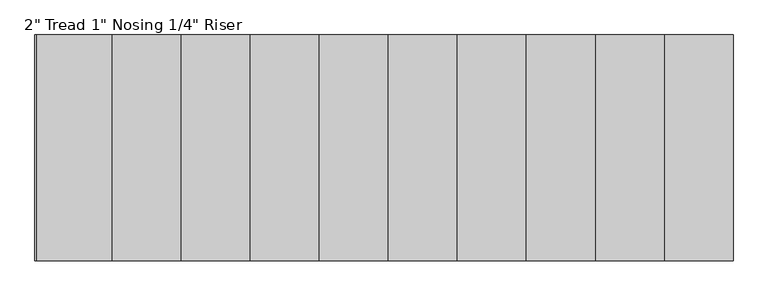
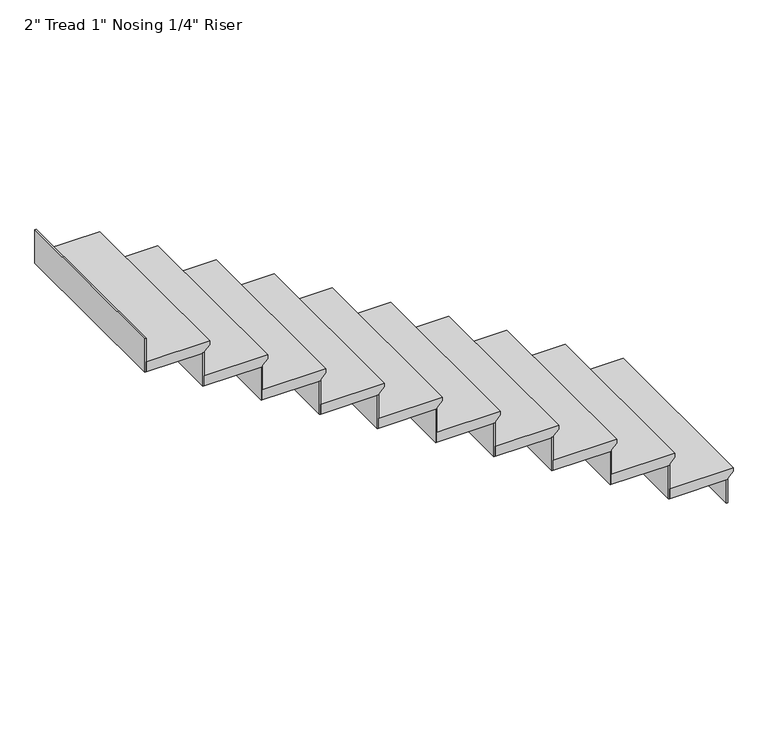
"""IFC4 building model written with IfcOpenShell, lengths in millimetres: stair flight geometry."""

from ifc_helpers import new_model, si_unit, origin, place, context, project, spatial, faceted_brep, source, transform, mapped, element, save


def stair_flight_4502834e(model_context):
    return source(origin(), model_context, "Body", "Brep", [
        faceted_brep([(-5990.8517085, 2919.0826226, 6855.8833333), (-5990.8517085, 2919.0826226, 6874.9333333), (-5990.8517085, 2004.6826226, 6874.9333333), (-5990.8517085, 2004.6826226, 6855.8833333), (-6016.2517085, 2919.0826226, 6830.4833333), (-6016.2517085, 2004.6826226, 6830.4833333), (-6295.6517085, 2919.0826226, 6874.9333333), (-6295.6517085, 2004.6826226, 6874.9333333), (-6016.2517085, 2004.6826226, 6824.1333333), (-6295.6517085, 2004.6826226, 6824.1333333), (-6295.6517085, 2919.0826226, 6824.1333333), (-6016.2517085, 2919.0826226, 6824.1333333)], [[[0, 1, 2, 3]], [[4, 0, 3, 5]], [[2, 1, 6, 7]], [[8, 9, 10, 11]], [[2, 7, 9, 8, 5, 3]], [[8, 11, 4, 5]], [[6, 1, 0, 4, 11, 10]], [[7, 6, 10, 9]]]),
        faceted_brep([(-6016.2517085, 2919.0826226, 6824.1333333), (-6016.2517085, 2919.0826226, 6705.6), (-6022.6017085, 2919.0826226, 6705.6), (-6022.6017085, 2919.0826226, 6824.1333333), (-6016.2517085, 2004.6826226, 6824.1333333), (-6022.6017085, 2004.6826226, 6824.1333333), (-6022.6017085, 2004.6826226, 6705.6), (-6016.2517085, 2004.6826226, 6705.6)], [[[0, 1, 2, 3]], [[4, 5, 6, 7]], [[1, 0, 4, 7]], [[2, 1, 7, 6]], [[3, 2, 6, 5]], [[0, 3, 5, 4]]]),
        faceted_brep([(-6295.6517085, 2919.0826226, 6993.4666667), (-6295.6517085, 2919.0826226, 6824.1333333), (-6302.0017085, 2919.0826226, 6824.1333333), (-6302.0017085, 2919.0826226, 6993.4666667), (-6295.6517085, 2004.6826226, 6993.4666667), (-6302.0017085, 2004.6826226, 6993.4666667), (-6302.0017085, 2004.6826226, 6824.1333333), (-6295.6517085, 2004.6826226, 6824.1333333)], [[[0, 1, 2, 3]], [[4, 5, 6, 7]], [[1, 0, 4, 7]], [[2, 1, 7, 6]], [[3, 2, 6, 5]], [[0, 3, 5, 4]]]),
        faceted_brep([(-6270.2517085, 2004.6826226, 7044.2666667), (-6270.2517085, 2919.0826226, 7044.2666667), (-6575.0517085, 2919.0826226, 7044.2666667), (-6575.0517085, 2004.6826226, 7044.2666667), (-6295.6517085, 2004.6826226, 6993.4666667), (-6575.0517085, 2004.6826226, 6993.4666667), (-6575.0517085, 2919.0826226, 6993.4666667), (-6295.6517085, 2919.0826226, 6993.4666667), (-6295.6517085, 2004.6826226, 6999.8166667), (-6270.2517085, 2004.6826226, 7025.2166667), (-6295.6517085, 2919.0826226, 6999.8166667), (-6270.2517085, 2919.0826226, 7025.2166667)], [[[0, 1, 2, 3]], [[4, 5, 6, 7]], [[0, 3, 5, 4, 8, 9]], [[4, 7, 10, 8]], [[2, 1, 11, 10, 7, 6]], [[3, 2, 6, 5]], [[11, 1, 0, 9]], [[10, 11, 9, 8]]]),
        faceted_brep([(-6575.0517085, 2919.0826226, 7162.8), (-6575.0517085, 2919.0826226, 6993.4666667), (-6581.4017085, 2919.0826226, 6993.4666667), (-6581.4017085, 2919.0826226, 7162.8), (-6575.0517085, 2004.6826226, 7162.8), (-6581.4017085, 2004.6826226, 7162.8), (-6581.4017085, 2004.6826226, 6993.4666667), (-6575.0517085, 2004.6826226, 6993.4666667)], [[[0, 1, 2, 3]], [[4, 5, 6, 7]], [[1, 0, 4, 7]], [[2, 1, 7, 6]], [[3, 2, 6, 5]], [[0, 3, 5, 4]]]),
        faceted_brep([(-6549.6517085, 2004.6826226, 7213.6), (-6549.6517085, 2919.0826226, 7213.6), (-6854.4517085, 2919.0826226, 7213.6), (-6854.4517085, 2004.6826226, 7213.6), (-6575.0517085, 2004.6826226, 7162.8), (-6854.4517085, 2004.6826226, 7162.8), (-6854.4517085, 2919.0826226, 7162.8), (-6575.0517085, 2919.0826226, 7162.8), (-6575.0517085, 2004.6826226, 7169.15), (-6549.6517085, 2004.6826226, 7194.55), (-6575.0517085, 2919.0826226, 7169.15), (-6549.6517085, 2919.0826226, 7194.55)], [[[0, 1, 2, 3]], [[4, 5, 6, 7]], [[0, 3, 5, 4, 8, 9]], [[4, 7, 10, 8]], [[2, 1, 11, 10, 7, 6]], [[3, 2, 6, 5]], [[11, 1, 0, 9]], [[10, 11, 9, 8]]]),
        faceted_brep([(-6854.4517085, 2919.0826226, 7332.1333333), (-6854.4517085, 2919.0826226, 7162.8), (-6860.8017085, 2919.0826226, 7162.8), (-6860.8017085, 2919.0826226, 7332.1333333), (-6854.4517085, 2004.6826226, 7332.1333333), (-6860.8017085, 2004.6826226, 7332.1333333), (-6860.8017085, 2004.6826226, 7162.8), (-6854.4517085, 2004.6826226, 7162.8)], [[[0, 1, 2, 3]], [[4, 5, 6, 7]], [[1, 0, 4, 7]], [[2, 1, 7, 6]], [[3, 2, 6, 5]], [[0, 3, 5, 4]]]),
        faceted_brep([(-6829.0517085, 2004.6826226, 7382.9333333), (-6829.0517085, 2919.0826226, 7382.9333333), (-7133.8517085, 2919.0826226, 7382.9333333), (-7133.8517085, 2004.6826226, 7382.9333333), (-6854.4517085, 2004.6826226, 7332.1333333), (-7133.8517085, 2004.6826226, 7332.1333333), (-7133.8517085, 2919.0826226, 7332.1333333), (-6854.4517085, 2919.0826226, 7332.1333333), (-6854.4517085, 2004.6826226, 7338.4833333), (-6829.0517085, 2004.6826226, 7363.8833333), (-6854.4517085, 2919.0826226, 7338.4833333), (-6829.0517085, 2919.0826226, 7363.8833333)], [[[0, 1, 2, 3]], [[4, 5, 6, 7]], [[0, 3, 5, 4, 8, 9]], [[4, 7, 10, 8]], [[2, 1, 11, 10, 7, 6]], [[3, 2, 6, 5]], [[11, 1, 0, 9]], [[10, 11, 9, 8]]]),
        faceted_brep([(-7133.8517085, 2919.0826226, 7501.4666667), (-7133.8517085, 2919.0826226, 7332.1333333), (-7140.2017085, 2919.0826226, 7332.1333333), (-7140.2017085, 2919.0826226, 7501.4666667), (-7133.8517085, 2004.6826226, 7501.4666667), (-7140.2017085, 2004.6826226, 7501.4666667), (-7140.2017085, 2004.6826226, 7332.1333333), (-7133.8517085, 2004.6826226, 7332.1333333)], [[[0, 1, 2, 3]], [[4, 5, 6, 7]], [[1, 0, 4, 7]], [[2, 1, 7, 6]], [[3, 2, 6, 5]], [[0, 3, 5, 4]]]),
        faceted_brep([(-7108.4517085, 2004.6826226, 7552.2666667), (-7108.4517085, 2919.0826226, 7552.2666667), (-7413.2517085, 2919.0826226, 7552.2666667), (-7413.2517085, 2004.6826226, 7552.2666667), (-7133.8517085, 2004.6826226, 7501.4666667), (-7413.2517085, 2004.6826226, 7501.4666667), (-7413.2517085, 2919.0826226, 7501.4666667), (-7133.8517085, 2919.0826226, 7501.4666667), (-7133.8517085, 2004.6826226, 7507.8166667), (-7108.4517085, 2004.6826226, 7533.2166667), (-7133.8517085, 2919.0826226, 7507.8166667), (-7108.4517085, 2919.0826226, 7533.2166667)], [[[0, 1, 2, 3]], [[4, 5, 6, 7]], [[0, 3, 5, 4, 8, 9]], [[4, 7, 10, 8]], [[2, 1, 11, 10, 7, 6]], [[3, 2, 6, 5]], [[11, 1, 0, 9]], [[10, 11, 9, 8]]]),
        faceted_brep([(-7413.2517085, 2919.0826226, 7670.8), (-7413.2517085, 2919.0826226, 7501.4666667), (-7419.6017085, 2919.0826226, 7501.4666667), (-7419.6017085, 2919.0826226, 7670.8), (-7413.2517085, 2004.6826226, 7670.8), (-7419.6017085, 2004.6826226, 7670.8), (-7419.6017085, 2004.6826226, 7501.4666667), (-7413.2517085, 2004.6826226, 7501.4666667)], [[[0, 1, 2, 3]], [[4, 5, 6, 7]], [[1, 0, 4, 7]], [[2, 1, 7, 6]], [[3, 2, 6, 5]], [[0, 3, 5, 4]]]),
        faceted_brep([(-7387.8517085, 2004.6826226, 7721.6), (-7387.8517085, 2919.0826226, 7721.6), (-7692.6517085, 2919.0826226, 7721.6), (-7692.6517085, 2004.6826226, 7721.6), (-7413.2517085, 2004.6826226, 7670.8), (-7692.6517085, 2004.6826226, 7670.8), (-7692.6517085, 2919.0826226, 7670.8), (-7413.2517085, 2919.0826226, 7670.8), (-7413.2517085, 2004.6826226, 7677.15), (-7387.8517085, 2004.6826226, 7702.55), (-7413.2517085, 2919.0826226, 7677.15), (-7387.8517085, 2919.0826226, 7702.55)], [[[0, 1, 2, 3]], [[4, 5, 6, 7]], [[0, 3, 5, 4, 8, 9]], [[4, 7, 10, 8]], [[2, 1, 11, 10, 7, 6]], [[3, 2, 6, 5]], [[11, 1, 0, 9]], [[10, 11, 9, 8]]]),
        faceted_brep([(-7692.6517085, 2919.0826226, 7840.1333333), (-7692.6517085, 2919.0826226, 7670.8), (-7699.0017085, 2919.0826226, 7670.8), (-7699.0017085, 2919.0826226, 7840.1333333), (-7692.6517085, 2004.6826226, 7840.1333333), (-7699.0017085, 2004.6826226, 7840.1333333), (-7699.0017085, 2004.6826226, 7670.8), (-7692.6517085, 2004.6826226, 7670.8)], [[[0, 1, 2, 3]], [[4, 5, 6, 7]], [[1, 0, 4, 7]], [[2, 1, 7, 6]], [[3, 2, 6, 5]], [[0, 3, 5, 4]]]),
        faceted_brep([(-7667.2517085, 2004.6826226, 7890.9333333), (-7667.2517085, 2919.0826226, 7890.9333333), (-7972.0517085, 2919.0826226, 7890.9333333), (-7972.0517085, 2004.6826226, 7890.9333333), (-7692.6517085, 2004.6826226, 7840.1333333), (-7972.0517085, 2004.6826226, 7840.1333333), (-7972.0517085, 2919.0826226, 7840.1333333), (-7692.6517085, 2919.0826226, 7840.1333333), (-7692.6517085, 2004.6826226, 7846.4833333), (-7667.2517085, 2004.6826226, 7871.8833333), (-7692.6517085, 2919.0826226, 7846.4833333), (-7667.2517085, 2919.0826226, 7871.8833333)], [[[0, 1, 2, 3]], [[4, 5, 6, 7]], [[0, 3, 5, 4, 8, 9]], [[4, 7, 10, 8]], [[2, 1, 11, 10, 7, 6]], [[3, 2, 6, 5]], [[11, 1, 0, 9]], [[10, 11, 9, 8]]]),
        faceted_brep([(-7972.0517085, 2919.0826226, 8009.4666667), (-7972.0517085, 2919.0826226, 7840.1333333), (-7978.4017085, 2919.0826226, 7840.1333333), (-7978.4017085, 2919.0826226, 8009.4666667), (-7972.0517085, 2004.6826226, 8009.4666667), (-7978.4017085, 2004.6826226, 8009.4666667), (-7978.4017085, 2004.6826226, 7840.1333333), (-7972.0517085, 2004.6826226, 7840.1333333)], [[[0, 1, 2, 3]], [[4, 5, 6, 7]], [[1, 0, 4, 7]], [[2, 1, 7, 6]], [[3, 2, 6, 5]], [[0, 3, 5, 4]]]),
        faceted_brep([(-7946.6517085, 2004.6826226, 8060.2666667), (-7946.6517085, 2919.0826226, 8060.2666667), (-8251.4517085, 2919.0826226, 8060.2666667), (-8251.4517085, 2004.6826226, 8060.2666667), (-7972.0517085, 2004.6826226, 8009.4666667), (-8251.4517085, 2004.6826226, 8009.4666667), (-8251.4517085, 2919.0826226, 8009.4666667), (-7972.0517085, 2919.0826226, 8009.4666667), (-7972.0517085, 2004.6826226, 8015.8166667), (-7946.6517085, 2004.6826226, 8041.2166667), (-7972.0517085, 2919.0826226, 8015.8166667), (-7946.6517085, 2919.0826226, 8041.2166667)], [[[0, 1, 2, 3]], [[4, 5, 6, 7]], [[0, 3, 5, 4, 8, 9]], [[4, 7, 10, 8]], [[2, 1, 11, 10, 7, 6]], [[3, 2, 6, 5]], [[11, 1, 0, 9]], [[10, 11, 9, 8]]]),
        faceted_brep([(-8251.4517085, 2919.0826226, 8178.8), (-8251.4517085, 2919.0826226, 8009.4666667), (-8257.8017085, 2919.0826226, 8009.4666667), (-8257.8017085, 2919.0826226, 8178.8), (-8251.4517085, 2004.6826226, 8178.8), (-8257.8017085, 2004.6826226, 8178.8), (-8257.8017085, 2004.6826226, 8009.4666667), (-8251.4517085, 2004.6826226, 8009.4666667)], [[[0, 1, 2, 3]], [[4, 5, 6, 7]], [[1, 0, 4, 7]], [[2, 1, 7, 6]], [[3, 2, 6, 5]], [[0, 3, 5, 4]]]),
        faceted_brep([(-8226.0517085, 2004.6826226, 8229.6), (-8226.0517085, 2919.0826226, 8229.6), (-8530.8517085, 2919.0826226, 8229.6), (-8530.8517085, 2004.6826226, 8229.6), (-8251.4517085, 2004.6826226, 8178.8), (-8530.8517085, 2004.6826226, 8178.8), (-8530.8517085, 2919.0826226, 8178.8), (-8251.4517085, 2919.0826226, 8178.8), (-8251.4517085, 2004.6826226, 8185.15), (-8226.0517085, 2004.6826226, 8210.55), (-8251.4517085, 2919.0826226, 8185.15), (-8226.0517085, 2919.0826226, 8210.55)], [[[0, 1, 2, 3]], [[4, 5, 6, 7]], [[0, 3, 5, 4, 8, 9]], [[4, 7, 10, 8]], [[2, 1, 11, 10, 7, 6]], [[3, 2, 6, 5]], [[11, 1, 0, 9]], [[10, 11, 9, 8]]]),
        faceted_brep([(-8810.2517085, 2919.0826226, 8517.4666667), (-8810.2517085, 2919.0826226, 8348.1333333), (-8816.6017085, 2919.0826226, 8348.1333333), (-8816.6017085, 2919.0826226, 8517.4666667), (-8810.2517085, 2004.6826226, 8517.4666667), (-8816.6017085, 2004.6826226, 8517.4666667), (-8816.6017085, 2004.6826226, 8348.1333333), (-8810.2517085, 2004.6826226, 8348.1333333)], [[[0, 1, 2, 3]], [[4, 5, 6, 7]], [[1, 0, 4, 7]], [[2, 1, 7, 6]], [[3, 2, 6, 5]], [[0, 3, 5, 4]]]),
        faceted_brep([(-8530.8517085, 2919.0826226, 8348.1333333), (-8530.8517085, 2919.0826226, 8178.8), (-8537.2017085, 2919.0826226, 8178.8), (-8537.2017085, 2919.0826226, 8348.1333333), (-8530.8517085, 2004.6826226, 8348.1333333), (-8537.2017085, 2004.6826226, 8348.1333333), (-8537.2017085, 2004.6826226, 8178.8), (-8530.8517085, 2004.6826226, 8178.8)], [[[0, 1, 2, 3]], [[4, 5, 6, 7]], [[1, 0, 4, 7]], [[2, 1, 7, 6]], [[3, 2, 6, 5]], [[0, 3, 5, 4]]]),
        faceted_brep([(-8505.4517085, 2004.6826226, 8398.9333333), (-8505.4517085, 2919.0826226, 8398.9333333), (-8784.8517085, 2919.0826226, 8398.9333333), (-8810.2517085, 2919.0826226, 8398.9333333), (-8810.2517085, 2004.6826226, 8398.9333333), (-8530.8517085, 2004.6826226, 8348.1333333), (-8810.2517085, 2004.6826226, 8348.1333333), (-8810.2517085, 2919.0826226, 8348.1333333), (-8784.8517085, 2919.0826226, 8348.1333333), (-8530.8517085, 2919.0826226, 8348.1333333), (-8530.8517085, 2004.6826226, 8354.4833333), (-8505.4517085, 2004.6826226, 8379.8833333), (-8530.8517085, 2919.0826226, 8354.4833333), (-8505.4517085, 2919.0826226, 8379.8833333)], [[[0, 1, 2, 3, 4]], [[5, 6, 7, 8, 9]], [[0, 4, 6, 5, 10, 11]], [[5, 9, 12, 10]], [[2, 1, 13, 12, 9, 8]], [[3, 2, 8, 7]], [[4, 3, 7, 6]], [[13, 1, 0, 11]], [[12, 13, 11, 10]]]),
    ])


if __name__ == "__main__":
    model = new_model("IFC4")
    model_context = context("Model", 3, world=origin())
    ifc_project = project(units=[si_unit("LENGTHUNIT", "METRE", prefix="MILLI")], contexts=[model_context])
    site = spatial("IfcSite", under=ifc_project)
    building = spatial("IfcBuilding", under=site)
    placement = place(None, origin())
    stair_flight_shape = stair_flight_4502834e(model_context)
    element("IfcStairFlight", 1, ObjectType="2\" Tread 1\" Nosing 1/4\" Riser", at=placement, inside=building, context=model_context, shape_type="MappedRepresentation", body=[
        mapped(stair_flight_shape, transform((0.0, 0.0, 0.0), x_axis=(1.0, 0.0, 0.0), y_axis=(0.0, 1.0, 0.0), z_axis=(0.0, 0.0, 1.0))),
    ])
    save(model, "model.ifc")
